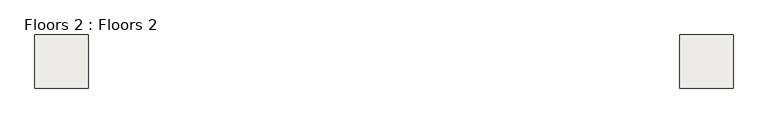
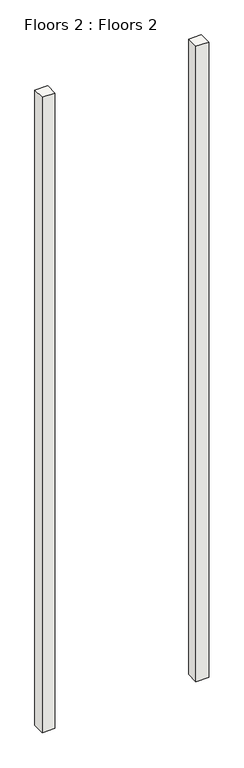
"""IFC4 building model written with IfcOpenShell, lengths in millimetres: slab geometry, Floors 2 : Floors 2."""

from ifc_helpers import new_model, si_unit, origin, origin_with_axes, place, context, project, spatial, polyline, outline, extrude, source, transform, mapped, element, save


def floors_2_floors_2_8417aeb3(model_context):
    return source(origin(), model_context, "Body", "SweptSolid", [
        extrude(outline(polyline([(-2616.758803, -1496.1217987), (-2845.358803, -1496.1217987), (-2845.358803, -1267.5217235), (-2616.758803, -1267.5217235), (-2616.758803, -1496.1217987)])), origin_with_axes(), (0.0, 0.0, 1.0), 12109.3035222),
        extrude(outline(polyline([(-76.758803, -1496.1217987), (-76.758803, -1267.5217987), (151.841197, -1267.5217987), (151.841197, -1496.1217987), (-76.758803, -1496.1217987)])), origin_with_axes(), (0.0, 0.0, 1.0), 12109.3035222),
    ])


if __name__ == "__main__":
    model = new_model("IFC4")
    model_context = context("Model", 3, world=origin())
    ifc_project = project(units=[si_unit("LENGTHUNIT", "METRE", prefix="MILLI")], contexts=[model_context])
    site = spatial("IfcSite", under=ifc_project)
    building = spatial("IfcBuilding", under=site)
    placement = place(None, origin())
    floors_2_floors_2_shape = floors_2_floors_2_8417aeb3(model_context)
    element("IfcSlab", 1, ObjectType="Floors 2 : Floors 2", at=placement, inside=building, context=model_context, shape_type="MappedRepresentation", body=[
        mapped(floors_2_floors_2_shape, transform((0.0, 0.0, 0.0), x_axis=(1.0, 0.0, 0.0), y_axis=(0.0, 1.0, 0.0), z_axis=(0.0, 0.0, 1.0))),
    ])
    save(model, "model.ifc")

# Revit data of these elements
# Element 1 (IfcSlab, "Floors 2 : Floors 2")
#   Materials on its faces: "Default Floor", "1 wood"
# Materials
#   "Default Floor": colour RGB 128 128 128, transparency 0, Cost = 0
#   "1 wood": class "Generic", colour RGB 61 46 37, transparency 0, Cost = 0
